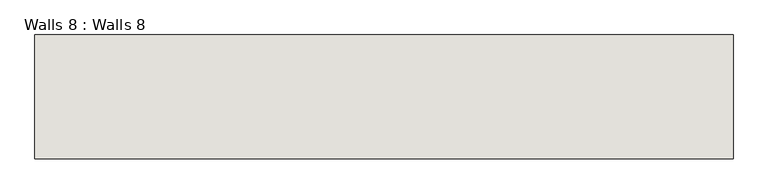
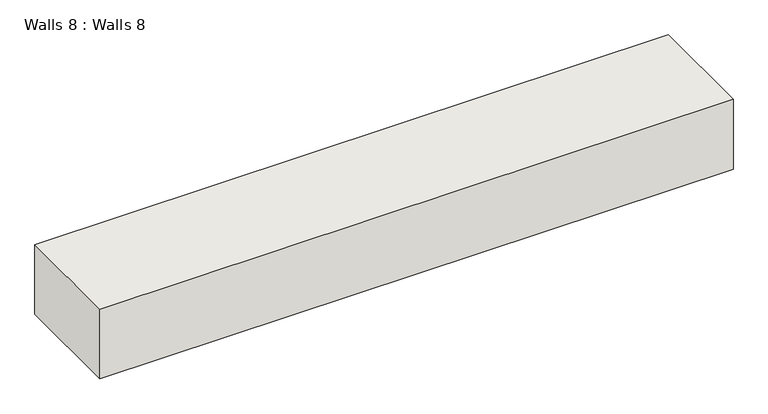
"""IFC4 building model written with IfcOpenShell, lengths in millimetres: wall geometry, Walls 8 : Walls 8."""

from ifc_helpers import new_model, si_unit, frame, origin, place, context, project, spatial, polyline, outline, extrude, source, transform, mapped, element, save


def walls_8_walls_8_87457aad(model_context):
    return source(origin(), model_context, "Body", "SweptSolid", [
        extrude(outline(polyline([(-6446.5718872, 3251.3956099), (-9880.3407032, 3251.3956099), (-9880.3407032, 3860.9956099), (-6446.5718872, 3860.9956099), (-6446.5718872, 3251.3956099)])), frame((0.0, 0.0, 5696.0), z_axis=(0.0, 0.0, 1.0), x_axis=(1.0, 0.0, 0.0)), (0.0, 0.0, 1.0), 400.0),
    ])


if __name__ == "__main__":
    model = new_model("IFC4")
    model_context = context("Model", 3, world=origin())
    ifc_project = project(units=[si_unit("LENGTHUNIT", "METRE", prefix="MILLI")], contexts=[model_context])
    site = spatial("IfcSite", under=ifc_project)
    building = spatial("IfcBuilding", under=site)
    placement = place(None, origin())
    walls_8_walls_8_shape = walls_8_walls_8_87457aad(model_context)
    element("IfcWall", 1, ObjectType="Walls 8 : Walls 8", at=placement, inside=building, context=model_context, shape_type="MappedRepresentation", body=[
        mapped(walls_8_walls_8_shape, transform((0.0, 0.0, 0.0), x_axis=(1.0, 0.0, 0.0), y_axis=(0.0, 1.0, 0.0), z_axis=(0.0, 0.0, 1.0))),
    ])
    save(model, "model.ifc")

# Revit data of these elements
# Element 1 (IfcWall, "Walls 8 : Walls 8")
#   Materials on its faces: "Default Wall"
# Materials
#   "Default Wall": colour RGB 80 80 80, transparency 0
